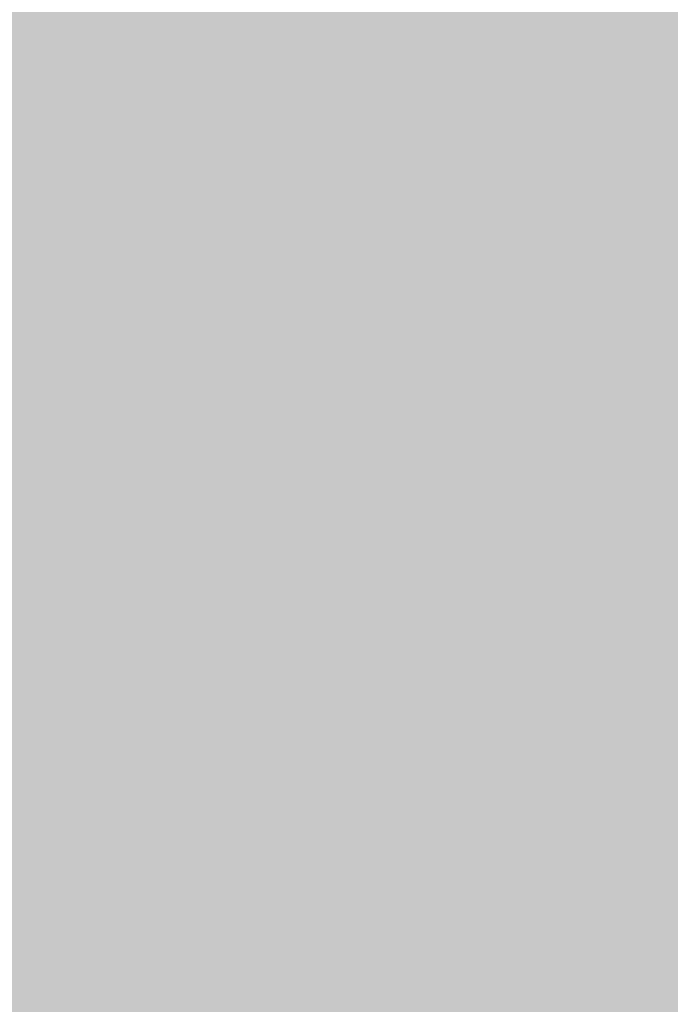
# Model space of a CAD drawing. Units: millimetres. Extents: x 0 to 2267, y 0 to 1823.
# Tile 43 of 256: x 1593.5605 to 1593.7801, y 1226.3857 to 1226.718. Entities that reach past the tile are written whole.
import ezdxf

# ---------------------------------------------------------------- set-up
doc = ezdxf.new("R2010")
doc.units = ezdxf.units.MM
doc.header["$MEASUREMENT"] = 0
doc.layers.add('M-HATC', color=252, linetype='Continuous', lineweight=18)

msp = doc.modelspace()

# ---------------------------------------------------------------- hatches: boundary and pattern name
at = {"layer": 'M-HATC'}
h = msp.add_hatch(color=256, dxfattribs=at)
h.dxf.hatch_style = 1
h.paths.add_polyline_path([(2055.77105, 1603.06204), (1381.08677, 1603.06204), (1381.08677, 1598.06204), (2055.77105, 1598.06204)])
h.paths.add_polyline_path([(2055.77105, 1598.06204), (1381.08677, 1598.06204), (1381.08677, 1593.06204), (2055.77105, 1593.06204)])
h.paths.add_polyline_path([(2051.30737, 1536.76088), (1385.55044, 1536.76088), (1385.55044, 1526.76088), (1387.55044, 1526.76088), (1388.53662, 1525.05276), (1385.33187, 1521.23348), (1385.33187, 1521.22256), (2050.25417, 1522.74913), (2048.32119, 1525.05276), (2049.30737, 1526.76088), (2051.30737, 1526.76088)])
edge = h.paths.add_edge_path()
edge.add_arc((1847.53451, 1379.14917), 135, 222.6030607, 222.8908505, ccw=False)
edge.add_line((1748.16629, 1287.76561), (1683.09212, 1287.76561))
edge.add_arc((1583.7239, 1379.14917), 135, 317.1091495, 317.3969393, ccw=False)
edge.add_arc((1678.9686, 1290.67067), 5, 222.89085, 317.10915, ccw=False)
edge.add_arc((1774.21331, 1379.14917), 135, 222.6030607, 222.8908505, ccw=False)
edge.add_line((1674.84509, 1287.76561), (1609.77092, 1287.76561))
edge.add_arc((1510.4027, 1379.14917), 135, 317.1091495, 317.3969393, ccw=False)
edge.add_arc((1605.6474, 1290.67067), 5, 222.89085, 317.10915, ccw=False)
edge.add_arc((1700.89211, 1379.14917), 135, 222.6030607, 222.8908505, ccw=False)
edge.add_line((1601.52388, 1287.76561), (1536.44972, 1287.76561))
edge.add_arc((1437.08149, 1379.14917), 135, 317.1091495, 317.3969393, ccw=False)
edge.add_arc((1532.3262, 1290.67067), 5, 222.89085, 317.10915, ccw=False)
edge.add_arc((1627.57091, 1379.14917), 135, 222.6030607, 222.8908505, ccw=False)
edge.add_line((1528.20268, 1287.76561), (1505.92891, 1287.76561))
edge.add_spline(control_points=[(1505.92891, 1287.76561), (1504.26224, 1287.76561), (1504.26224, 1282.76561), (1505.92891, 1282.76561)], knot_values=[0, 0, 0, 0, 5, 5, 5, 5], degree=3, periodic=0)
edge.add_line((1505.92891, 1282.76561), (1930.92891, 1282.76561))
edge.add_spline(control_points=[(1930.92891, 1282.76561), (1932.59557, 1282.76561), (1932.59557, 1287.76561), (1930.92891, 1287.76561)], knot_values=[0, 0, 0, 0, 5, 5, 5, 5], degree=3, periodic=0)
edge.add_line((1930.92891, 1287.76561), (1903.05573, 1287.76561))
edge.add_arc((1803.6875, 1379.14917), 135, 317.1091495, 317.3969393, ccw=False)
edge.add_arc((1898.93221, 1290.67067), 5, 222.89085, 317.10915, ccw=False)
edge.add_arc((1994.17691, 1379.14917), 135, 222.6030607, 222.8908505, ccw=False)
edge.add_line((1894.80869, 1287.76561), (1829.73452, 1287.76561))
edge.add_arc((1730.3663, 1379.14917), 135, 317.1091495, 317.3969393, ccw=False)
edge.add_arc((1825.61101, 1290.67067), 5, 222.89085, 317.10915, ccw=False)
edge.add_arc((1920.85571, 1379.14917), 135, 222.6030607, 222.8908505, ccw=False)
edge.add_line((1821.48749, 1287.76561), (1756.41332, 1287.76561))
edge.add_arc((1657.0451, 1379.14917), 135, 317.1091495, 317.3969393, ccw=False)
edge.add_arc((1752.28981, 1290.67067), 5, 222.89085, 317.10915, ccw=False)
edge = h.paths.add_edge_path()
edge.add_spline(control_points=[(1843.42891, 1227.24746), (1845.09557, 1227.24746), (1845.09557, 1232.24746), (1843.42891, 1232.24746)], knot_values=[0, 0, 0, 0, 5, 5, 5, 5], degree=3, periodic=0)
edge.add_line((1843.42891, 1232.24746), (1593.42891, 1232.24746))
edge.add_spline(control_points=[(1593.42891, 1232.24746), (1591.76224, 1232.24746), (1591.76224, 1227.24746), (1593.42891, 1227.24746)], knot_values=[0, 0, 0, 0, 5, 5, 5, 5], degree=3, periodic=0)
edge.add_line((1593.42891, 1227.24746), (1843.42891, 1227.24746))
h.paths.add_polyline_path([(1905.92891, 1127.41706), (1530.92891, 1127.41706, 0.414214), (1520.92891, 1117.41706), (1530.92891, 1117.41706), (1915.92891, 1117.41706, 0.414214)])
edge = h.paths.add_edge_path()
edge.add_arc((1397.08577, 1498.40775), 12.72993, 90.782146, 190.878706, ccw=False)
edge.add_line((1396.912, 1511.13649), (1428.00968, 1511.34875))
edge.add_line((1428.00968, 1511.34875), (1433.00968, 1511.34875))
edge.add_line((1433.00968, 1511.34875), (1434.439, 1511.34875))
edge.add_arc((1419.474, 1498.08041), 20, 41.560995, 74.082109)
edge.add_line((1424.95919, 1517.31353), (1399.93509, 1517.25608))
edge.add_spline(control_points=[(1399.93074, 1517.25607), (1399.88398, 1517.21312), (1399.8328, 1517.16893), (1399.77741, 1517.1236)], knot_values=[11.567499, 11.567499, 11.567499, 11.567499, 11.814249, 11.814249, 11.814249, 11.814249], degree=3, periodic=0)
edge.add_spline(control_points=[(1399.63279, 1517.00986), (1399.58305, 1516.97214), (1399.53072, 1516.93375), (1399.47591, 1516.89474)], knot_values=[11.167718, 11.167718, 11.167718, 11.167718, 11.365188, 11.365188, 11.365188, 11.365188], degree=3, periodic=0)
edge.add_spline(control_points=[(1399.33981, 1516.80007), (1399.15144, 1516.67185), (1398.93836, 1516.5377), (1398.70404, 1516.39942)], knot_values=[10.376405, 10.376405, 10.376405, 10.376405, 11.00994, 11.00994, 11.00994, 11.00994], degree=3, periodic=0)
edge.add_spline(control_points=[(1398.65716, 1516.37187), (1398.57885, 1516.32602), (1398.49825, 1516.27974), (1398.41549, 1516.23309)], knot_values=[10.125175, 10.125175, 10.125175, 10.125175, 10.334406, 10.334406, 10.334406, 10.334406], degree=3, periodic=0)
edge.add_spline(control_points=[(1398.26422, 1516.14874), (1398.19595, 1516.11107), (1398.12634, 1516.07319), (1398.05546, 1516.03513)], knot_values=[9.832246, 9.832246, 9.832246, 9.832246, 9.999658, 9.999658, 9.999658, 9.999658], degree=3, periodic=0)
edge.add_spline(control_points=[(1397.9987, 1516.00476), (1397.73115, 1515.86211), (1397.44602, 1515.71707), (1397.14664, 1515.57138)], knot_values=[9.161808, 9.161808, 9.161808, 9.161808, 9.787769, 9.787769, 9.787769, 9.787769], degree=3, periodic=0)
edge.add_spline(control_points=[(1397.14664, 1515.57138), (1396.84182, 1515.42305), (1396.52223, 1515.27404), (1396.1914, 1515.12621)], knot_values=[8.524455, 8.524455, 8.524455, 8.524455, 9.161808, 9.161808, 9.161808, 9.161808], degree=3, periodic=0)
edge.add_spline(control_points=[(1396.07771, 1515.07565), (1395.98538, 1515.03478), (1395.89222, 1514.99402), (1395.7983, 1514.9534)], knot_values=[8.275193, 8.275193, 8.275193, 8.275193, 8.451726, 8.451726, 8.451726, 8.451726], degree=3, periodic=0)
edge.add_spline(control_points=[(1395.60184, 1514.86912), (1395.49975, 1514.82568), (1395.39685, 1514.78244), (1395.29322, 1514.73944)], knot_values=[7.962917, 7.962917, 7.962917, 7.962917, 8.152764, 8.152764, 8.152764, 8.152764], degree=3, periodic=0)
edge.add_spline(control_points=[(1395.21158, 1514.70568), (1394.82779, 1514.5475), (1394.43452, 1514.39287), (1394.03645, 1514.24422)], knot_values=[7.21254, 7.21254, 7.21254, 7.21254, 7.913148, 7.913148, 7.913148, 7.913148], degree=3, periodic=0)
edge.add_spline(control_points=[(1394.03645, 1514.24422), (1393.70758, 1514.12142), (1393.37544, 1514.0027), (1393.04267, 1513.88945)], knot_values=[6.633733, 6.633733, 6.633733, 6.633733, 7.21254, 7.21254, 7.21254, 7.21254], degree=3, periodic=0)
edge.add_spline(control_points=[(1392.82142, 1513.81499), (1392.71978, 1513.78118), (1392.61815, 1513.74791), (1392.51658, 1513.71521)], knot_values=[6.328796, 6.328796, 6.328796, 6.328796, 6.505493, 6.505493, 6.505493, 6.505493], degree=3, periodic=0)
edge.add_spline(control_points=[(1392.51658, 1513.71521), (1392.31873, 1513.65151), (1392.12116, 1513.59001), (1391.92441, 1513.53098)], knot_values=[5.984605, 5.984605, 5.984605, 5.984605, 6.328796, 6.328796, 6.328796, 6.328796], degree=3, periodic=0)
edge.add_spline(control_points=[(1391.79155, 1513.49146), (1391.31215, 1513.35011), (1390.83842, 1513.22392), (1390.37844, 1513.11711)], knot_values=[5.066697, 5.066697, 5.066697, 5.066697, 5.907055, 5.907055, 5.907055, 5.907055], degree=3, periodic=0)
edge.add_spline(control_points=[(1390.37844, 1513.11711), (1390.17973, 1513.07097), (1389.98359, 1513.02845), (1389.79067, 1512.98988)], knot_values=[4.70367, 4.70367, 4.70367, 4.70367, 5.066695, 5.066695, 5.066695, 5.066695], degree=3, periodic=0)
edge.add_spline(control_points=[(1389.42203, 1512.92036), (1389.24588, 1512.88922), (1389.0729, 1512.86172), (1388.90364, 1512.83814)], knot_values=[4.130571, 4.130571, 4.130571, 4.130571, 4.469816, 4.469816, 4.469816, 4.469816], degree=3, periodic=0)
edge.add_spline(control_points=[(1388.90364, 1512.83814), (1388.59103, 1512.7946), (1388.29108, 1512.76444), (1388.00714, 1512.74941)], knot_values=[3.504031, 3.504031, 3.504031, 3.504031, 4.130571, 4.130571, 4.130571, 4.130571], degree=3, periodic=0)
edge.add_spline(control_points=[(1387.9356, 1512.74593), (1387.85378, 1512.74231), (1387.77334, 1512.73997), (1387.69435, 1512.73898)], knot_values=[3.268866, 3.268866, 3.268866, 3.268866, 3.451164, 3.451164, 3.451164, 3.451164], degree=3, periodic=0)
edge.add_spline(control_points=[(1387.33512, 1512.74426), (1387.20757, 1512.74991), (1387.08472, 1512.7597), (1386.96699, 1512.77385)], knot_values=[2.670686, 2.670686, 2.670686, 2.670686, 2.984, 2.984, 2.984, 2.984], degree=3, periodic=0)
edge.add_spline(control_points=[(1386.83274, 1512.79225), (1386.82093, 1512.79407), (1386.80917, 1512.79594), (1386.79747, 1512.79787)], knot_values=[2.516981, 2.516981, 2.516981, 2.516981, 2.549528, 2.549528, 2.549528, 2.549528], degree=3, periodic=0)
edge.add_spline(control_points=[(1386.45257, 1512.87348), (1386.42573, 1512.88105), (1386.39931, 1512.88895), (1386.3733, 1512.89719)], knot_values=[2.095869, 2.095869, 2.095869, 2.095869, 2.17941, 2.17941, 2.17941, 2.17941], degree=3, periodic=0)
edge.add_spline(control_points=[(1386.06911, 1513.01889), (1386.06338, 1513.02174), (1386.05768, 1513.02463), (1386.05201, 1513.02753)], knot_values=[1.72453, 1.72453, 1.72453, 1.72453, 1.745933, 1.745933, 1.745933, 1.745933], degree=3, periodic=0)
edge.add_arc((1399.474, 1498.08041), 20, 131.824322, 180)
edge.add_arc((1630.33362, 1505.54843), 250.97076, 181.7051759, 236.427975)
edge.add_arc((1605.33992, 1483.30441), 218.7822, 238.660829, 243.3496099)
edge.add_arc((1647.09105, 1510.35917), 262.89859, 183.1298361, 237.8534422, ccw=False)
h.paths.add_polyline_path([(1406.53685, 1391.96444, 0.149382), (1491.55061, 1296.44177, -0.129517)], flags=17)
edge = h.paths.add_edge_path()
edge.add_arc((2037.38381, 1498.08041), 20, 0, 48.265868)
edge.add_spline(control_points=[(2050.69731, 1513.00525), (2050.65121, 1512.98471), (2050.60338, 1512.96554), (2050.55388, 1512.94771)], knot_values=[1.835652, 1.835652, 1.835652, 1.835652, 2.000781, 2.000781, 2.000781, 2.000781], degree=3, periodic=0)
edge.add_spline(control_points=[(2050.46156, 1512.91661), (2050.479, 1512.9221), (2050.49625, 1512.92774), (2050.51332, 1512.93353)], knot_values=[2.045477, 2.045477, 2.045477, 2.045477, 2.101389, 2.101389, 2.101389, 2.101389], degree=3, periodic=0)
edge.add_spline(control_points=[(2050.12896, 1512.83416), (2050.19843, 1512.84734), (2050.26573, 1512.86233), (2050.33075, 1512.87919)], knot_values=[2.237629, 2.237629, 2.237629, 2.237629, 2.435841, 2.435841, 2.435841, 2.435841], degree=3, periodic=0)
edge.add_spline(control_points=[(2050.09463, 1512.82783), (2050.10613, 1512.82989), (2050.11757, 1512.832), (2050.12896, 1512.83416)], knot_values=[2.435841, 2.435841, 2.435841, 2.435841, 2.468321, 2.468321, 2.468321, 2.468321], degree=3, periodic=0)
edge.add_spline(control_points=[(2049.78433, 1512.78511), (2049.85521, 1512.79219), (2049.92435, 1512.80077), (2049.99166, 1512.81088)], knot_values=[2.563852, 2.563852, 2.563852, 2.563852, 2.748541, 2.748541, 2.748541, 2.748541], degree=3, periodic=0)
edge.add_spline(control_points=[(2049.4052, 1512.76169), (2049.5364, 1512.76526), (2049.66292, 1512.77299), (2049.78433, 1512.78511)], knot_values=[2.748541, 2.748541, 2.748541, 2.748541, 3.064882, 3.064882, 3.064882, 3.064882], degree=3, periodic=0)
edge.add_spline(control_points=[(2049.16976, 1512.75968), (2049.23364, 1512.7591), (2049.29654, 1512.7594), (2049.35844, 1512.7606)], knot_values=[3.102309, 3.102309, 3.102309, 3.102309, 3.2503, 3.2503, 3.2503, 3.2503], degree=3, periodic=0)
edge.add_spline(control_points=[(2048.85727, 1512.76911), (2048.96378, 1512.76378), (2049.068, 1512.76061), (2049.16976, 1512.75968)], knot_values=[3.2503, 3.2503, 3.2503, 3.2503, 3.486069, 3.486069, 3.486069, 3.486069], degree=3, periodic=0)
edge.add_spline(control_points=[(2048.69241, 1512.77892), (2048.3729, 1512.80093), (2048.0345, 1512.84106), (2047.68175, 1512.89697)], knot_values=[3.606429, 3.606429, 3.606429, 3.606429, 4.2989, 4.2989, 4.2989, 4.2989], degree=3, periodic=0)
edge.add_spline(control_points=[(2047.68175, 1512.89697), (2047.5458, 1512.91852), (2047.40772, 1512.94241), (2047.26776, 1512.96851)], knot_values=[4.2989, 4.2989, 4.2989, 4.2989, 4.565769, 4.565769, 4.565769, 4.565769], degree=3, periodic=0)
edge.add_spline(control_points=[(2047.26776, 1512.96851), (2047.14494, 1512.99141), (2047.02067, 1513.01601), (2046.89514, 1513.04223)], knot_values=[4.565769, 4.565769, 4.565769, 4.565769, 4.799971, 4.799971, 4.799971, 4.799971], degree=3, periodic=0)
edge.add_spline(control_points=[(2046.89514, 1513.04223), (2046.52865, 1513.11875), (2046.15135, 1513.20899), (2045.7676, 1513.31068)], knot_values=[4.799971, 4.799971, 4.799971, 4.799971, 5.483718, 5.483718, 5.483718, 5.483718], degree=3, periodic=0)
edge.add_spline(control_points=[(2045.7676, 1513.31068), (2045.3724, 1513.41539), (2044.97036, 1513.53225), (2044.56625, 1513.65876)], knot_values=[5.483718, 5.483718, 5.483718, 5.483718, 6.187866, 6.187866, 6.187866, 6.187866], degree=3, periodic=0)
edge.add_spline(control_points=[(2044.56625, 1513.65876), (2044.41491, 1513.70614), (2044.26329, 1513.75487), (2044.11163, 1513.80482)], knot_values=[6.187866, 6.187866, 6.187866, 6.187866, 6.451551, 6.451551, 6.451551, 6.451551], degree=3, periodic=0)
edge.add_spline(control_points=[(2044.11163, 1513.80482), (2043.99666, 1513.84269), (2043.88167, 1513.88126), (2043.76676, 1513.92048)], knot_values=[6.451551, 6.451551, 6.451551, 6.451551, 6.651434, 6.651434, 6.651434, 6.651434], degree=3, periodic=0)
edge.add_spline(control_points=[(2043.76676, 1513.92048), (2043.37157, 1514.05536), (2042.97738, 1514.19789), (2042.58863, 1514.34575)], knot_values=[6.651434, 6.651434, 6.651434, 6.651434, 7.338879, 7.338879, 7.338879, 7.338879], degree=3, periodic=0)
edge.add_spline(control_points=[(2042.58863, 1514.34575), (2042.16431, 1514.50715), (2041.74647, 1514.67491), (2041.34086, 1514.84603)], knot_values=[7.338879, 7.338879, 7.338879, 7.338879, 8.089209, 8.089209, 8.089209, 8.089209], degree=3, periodic=0)
edge.add_spline(control_points=[(2041.34086, 1514.84603), (2041.1028, 1514.94647), (2040.86896, 1515.04806), (2040.64049, 1515.1502)], knot_values=[8.089209, 8.089209, 8.089209, 8.089209, 8.529587, 8.529587, 8.529587, 8.529587], degree=3, periodic=0)
edge.add_spline(control_points=[(2040.50999, 1515.20887), (2040.08238, 1515.40218), (2039.67475, 1515.59705), (2039.29495, 1515.78939)], knot_values=[8.613818, 8.613818, 8.613818, 8.613818, 9.44571, 9.44571, 9.44571, 9.44571], degree=3, periodic=0)
edge.add_spline(control_points=[(2039.29495, 1515.78939), (2039.0618, 1515.90746), (2038.83914, 1516.02458), (2038.62878, 1516.1398)], knot_values=[9.44571, 9.44571, 9.44571, 9.44571, 9.956404, 9.956404, 9.956404, 9.956404], degree=3, periodic=0)
edge.add_spline(control_points=[(2038.62878, 1516.1398), (2038.51874, 1516.20007), (2038.41207, 1516.25982), (2038.30903, 1516.31891)], knot_values=[9.956404, 9.956404, 9.956404, 9.956404, 10.223542, 10.223542, 10.223542, 10.223542], degree=3, periodic=0)
edge.add_spline(control_points=[(2038.30903, 1516.31891), (2038.21377, 1516.37354), (2038.12161, 1516.42762), (2038.03275, 1516.48102)], knot_values=[10.223542, 10.223542, 10.223542, 10.223542, 10.47051, 10.47051, 10.47051, 10.47051], degree=3, periodic=0)
edge.add_spline(control_points=[(2038.03275, 1516.48102), (2037.78552, 1516.62961), (2037.56388, 1516.77304), (2037.37225, 1516.909)], knot_values=[10.47051, 10.47051, 10.47051, 10.47051, 11.15767, 11.15767, 11.15767, 11.15767], degree=3, periodic=0)
edge.add_spline(control_points=[(2037.37225, 1516.909), (2037.27893, 1516.9752), (2037.19274, 1517.03963), (2037.11417, 1517.10203)], knot_values=[11.15767, 11.15767, 11.15767, 11.15767, 11.49227, 11.49227, 11.49227, 11.49227], degree=3, periodic=0)
edge.add_spline(control_points=[(2036.85638, 1517.32585), (2036.91481, 1517.26923), (2036.98143, 1517.21027), (2037.05573, 1517.14922)], knot_values=[11.577341, 11.577341, 11.577341, 11.577341, 11.91035, 11.91035, 11.91035, 11.91035], degree=3, periodic=0)
edge.add_spline(control_points=[(2036.80739, 1517.37475), (2036.82301, 1517.35865), (2036.83935, 1517.34235), (2036.85638, 1517.32585)], knot_values=[11.91035, 11.91035, 11.91035, 11.91035, 12.007402, 12.007402, 12.007402, 12.007402], degree=3, periodic=0)
edge.add_spline(control_points=[(2036.70167, 1517.494), (2036.71042, 1517.48299), (2036.71958, 1517.47185), (2036.72913, 1517.4606)], knot_values=[12.184155, 12.184155, 12.184155, 12.184155, 12.255409, 12.255409, 12.255409, 12.255409], degree=3, periodic=0)
edge.add_spline(control_points=[(2036.6159, 1517.6205), (2036.61998, 1517.61304), (2036.6243, 1517.6055), (2036.62885, 1517.59789)], knot_values=[12.487913, 12.487913, 12.487913, 12.487913, 12.541035, 12.541035, 12.541035, 12.541035], degree=3, periodic=0)
edge.add_spline(control_points=[(2036.56349, 1517.78599), (2036.56372, 1517.77936), (2036.56423, 1517.77264), (2036.56502, 1517.76582)], knot_values=[12.911761, 12.911761, 12.911761, 12.911761, 12.968286, 12.968286, 12.968286, 12.968286], degree=3, periodic=0)
edge.add_spline(control_points=[(2036.61663, 1517.93042), (2036.61248, 1517.92586), (2036.60857, 1517.92121), (2036.60491, 1517.91648)], knot_values=[13.382527, 13.382527, 13.382527, 13.382527, 13.433791, 13.433791, 13.433791, 13.433791], degree=3, periodic=0)
edge.add_spline(control_points=[(2036.74902, 1518.01695), (2036.73613, 1518.0116), (2036.72393, 1518.00601), (2036.71242, 1518.00018)], knot_values=[13.726299, 13.726299, 13.726299, 13.726299, 13.809928, 13.809928, 13.809928, 13.809928], degree=3, periodic=0)
edge.add_spline(control_points=[(2036.86043, 1518.05285), (2036.83863, 1518.04743), (2036.81809, 1518.04156), (2036.79879, 1518.03526)], knot_values=[13.910887, 13.910887, 13.910887, 13.910887, 14.02153, 14.02153, 14.02153, 14.02153], degree=3, periodic=0)
edge.add_line((2036.96387, 1518.08041), (2032.38381, 1518.08041))
edge.add_line((2032.38381, 1518.08041), (2027.38381, 1518.08041))
edge.add_line((2027.38381, 1518.08041), (2022.38381, 1518.08041))
edge.add_line((2022.38381, 1518.08041), (2017.38381, 1518.08041))
edge.add_arc((2017.38381, 1498.08041), 20, 90, 138.439005)
edge.add_line((2002.41881, 1511.34875), (2003.84813, 1511.34875))
edge.add_line((2003.84813, 1511.34875), (2008.84813, 1511.34875))
edge.add_line((2008.84813, 1511.34875), (2039.77204, 1511.13768))
edge.add_arc((2039.77204, 1498.40775), 12.72993, -10.878706, 90, ccw=False)
edge.add_arc((1789.76676, 1510.35917), 262.89859, 302.1465578, 356.8701639, ccw=False)
edge.add_arc((1831.51789, 1483.30441), 218.7822, 296.6503901, 301.339171)
edge.add_arc((1806.52419, 1505.54843), 250.97076, 303.572025, 358.2948241)
h.paths.add_polyline_path([(2030.32096, 1391.96444, -0.129517), (1945.3072, 1296.44177, 0.149382)], flags=17)
edge = h.paths.add_edge_path()
edge.add_spline(control_points=[(2037.2464, 1518.08209), (2037.28977, 1518.08098), (2037.33555, 1518.08041), (2037.3838, 1518.08041)], knot_values=[0.000012, 0.000012, 0.000012, 0.000012, 0.144754, 0.144754, 0.144754, 0.144754], degree=3, periodic=0)
edge.add_line((2037.33571, 1518.08041), (2037.00963, 1518.08041))
edge.add_spline(control_points=[(2037.00963, 1518.08041), (2036.98217, 1518.07678), (2036.95605, 1518.07266), (2036.93124, 1518.06808)], knot_values=[14.13465, 14.13465, 14.13465, 14.13465, 14.247197, 14.247197, 14.247197, 14.247197], degree=3, periodic=0)
edge.add_spline(control_points=[(2036.93124, 1518.06808), (2036.92764, 1518.06741), (2036.92407, 1518.06674), (2036.92053, 1518.06605)], knot_values=[14.118315, 14.118315, 14.118315, 14.118315, 14.13465, 14.13465, 14.13465, 14.13465], degree=3, periodic=0)
edge.add_spline(control_points=[(2036.92053, 1518.06605), (2036.9118, 1518.06436), (2036.90323, 1518.06262), (2036.89484, 1518.06081)], knot_values=[14.078086, 14.078086, 14.078086, 14.078086, 14.118315, 14.118315, 14.118315, 14.118315], degree=3, periodic=0)
edge.add_spline(control_points=[(2036.89484, 1518.06081), (2036.88304, 1518.05827), (2036.87157, 1518.05562), (2036.86043, 1518.05285)], knot_values=[14.02153, 14.02153, 14.02153, 14.02153, 14.078086, 14.078086, 14.078086, 14.078086], degree=3, periodic=0)
edge.add_spline(control_points=[(2036.86043, 1518.05285), (2036.83863, 1518.04743), (2036.81809, 1518.04156), (2036.79879, 1518.03526)], knot_values=[13.910887, 13.910887, 13.910887, 13.910887, 14.02153, 14.02153, 14.02153, 14.02153], degree=3, periodic=0)
edge.add_spline(control_points=[(2036.79879, 1518.03526), (2036.79809, 1518.03504), (2036.7974, 1518.03481), (2036.79671, 1518.03458)], knot_values=[13.906906, 13.906906, 13.906906, 13.906906, 13.910887, 13.910887, 13.910887, 13.910887], degree=3, periodic=0)
edge.add_spline(control_points=[(2036.79671, 1518.03458), (2036.78819, 1518.03178), (2036.77991, 1518.02888), (2036.77187, 1518.02591)], knot_values=[13.857826, 13.857826, 13.857826, 13.857826, 13.906906, 13.906906, 13.906906, 13.906906], degree=3, periodic=0)
edge.add_spline(control_points=[(2036.77187, 1518.02591), (2036.76402, 1518.023), (2036.75641, 1518.02002), (2036.74902, 1518.01695)], knot_values=[13.809928, 13.809928, 13.809928, 13.809928, 13.857826, 13.857826, 13.857826, 13.857826], degree=3, periodic=0)
edge.add_spline(control_points=[(2036.74902, 1518.01695), (2036.73613, 1518.0116), (2036.72393, 1518.00601), (2036.71242, 1518.00018)], knot_values=[13.726299, 13.726299, 13.726299, 13.726299, 13.809928, 13.809928, 13.809928, 13.809928], degree=3, periodic=0)
edge.add_spline(control_points=[(2036.71242, 1518.00018), (2036.71211, 1518.00002), (2036.71179, 1517.99986), (2036.71147, 1517.99969)], knot_values=[13.723993, 13.723993, 13.723993, 13.723993, 13.726299, 13.726299, 13.726299, 13.726299], degree=3, periodic=0)
edge.add_spline(control_points=[(2036.71147, 1517.99969), (2036.70634, 1517.99708), (2036.70134, 1517.99441), (2036.69648, 1517.9917)], knot_values=[13.686536, 13.686536, 13.686536, 13.686536, 13.723993, 13.723993, 13.723993, 13.723993], degree=3, periodic=0)
edge.add_spline(control_points=[(2036.69648, 1517.9917), (2036.6919, 1517.98914), (2036.68744, 1517.98654), (2036.6831, 1517.9839)], knot_values=[13.651251, 13.651251, 13.651251, 13.651251, 13.686536, 13.686536, 13.686536, 13.686536], degree=3, periodic=0)
edge.add_spline(control_points=[(2036.6831, 1517.9839), (2036.67641, 1517.97983), (2036.67001, 1517.97566), (2036.6639, 1517.97139)], knot_values=[13.596804, 13.596804, 13.596804, 13.596804, 13.651251, 13.651251, 13.651251, 13.651251], degree=3, periodic=0)
edge.add_spline(control_points=[(2036.6639, 1517.97139), (2036.66358, 1517.97117), (2036.66326, 1517.97094), (2036.66294, 1517.97072)], knot_values=[13.593956, 13.593956, 13.593956, 13.593956, 13.596804, 13.596804, 13.596804, 13.596804], degree=3, periodic=0)
edge.add_spline(control_points=[(2036.66294, 1517.97072), (2036.6603, 1517.96886), (2036.65771, 1517.96698), (2036.65518, 1517.96509)], knot_values=[13.570322, 13.570322, 13.570322, 13.570322, 13.593956, 13.593956, 13.593956, 13.593956], degree=3, periodic=0)
edge.add_spline(control_points=[(2036.65518, 1517.96509), (2036.65251, 1517.9631), (2036.64991, 1517.96108), (2036.64737, 1517.95905)], knot_values=[13.545477, 13.545477, 13.545477, 13.545477, 13.570322, 13.570322, 13.570322, 13.570322], degree=3, periodic=0)
edge.add_spline(control_points=[(2036.64737, 1517.95905), (2036.64721, 1517.95892), (2036.64705, 1517.9588), (2036.64689, 1517.95867)], knot_values=[13.543931, 13.543931, 13.543931, 13.543931, 13.545477, 13.545477, 13.545477, 13.545477], degree=3, periodic=0)
edge.add_spline(control_points=[(2036.64689, 1517.95867), (2036.64121, 1517.95411), (2036.63582, 1517.94945), (2036.63073, 1517.94468)], knot_values=[13.488237, 13.488237, 13.488237, 13.488237, 13.543931, 13.543931, 13.543931, 13.543931], degree=3, periodic=0)
edge.add_spline(control_points=[(2036.63073, 1517.94468), (2036.62817, 1517.94229), (2036.62569, 1517.93988), (2036.62329, 1517.93744)], knot_values=[13.460307, 13.460307, 13.460307, 13.460307, 13.488237, 13.488237, 13.488237, 13.488237], degree=3, periodic=0)
edge.add_spline(control_points=[(2036.62329, 1517.93744), (2036.62151, 1517.93564), (2036.61978, 1517.93383), (2036.61809, 1517.932)], knot_values=[13.439712, 13.439712, 13.439712, 13.439712, 13.460307, 13.460307, 13.460307, 13.460307], degree=3, periodic=0)
edge.add_spline(control_points=[(2036.61809, 1517.932), (2036.6176, 1517.93147), (2036.61711, 1517.93095), (2036.61663, 1517.93042)], knot_values=[13.433791, 13.433791, 13.433791, 13.433791, 13.439712, 13.439712, 13.439712, 13.439712], degree=3, periodic=0)
edge.add_spline(control_points=[(2036.61663, 1517.93042), (2036.61248, 1517.92586), (2036.60857, 1517.92121), (2036.60491, 1517.91648)], knot_values=[13.382527, 13.382527, 13.382527, 13.382527, 13.433791, 13.433791, 13.433791, 13.433791], degree=3, periodic=0)
edge.add_spline(control_points=[(2036.60491, 1517.91648), (2036.60258, 1517.91347), (2036.60036, 1517.91044), (2036.59824, 1517.90737)], knot_values=[13.350017, 13.350017, 13.350017, 13.350017, 13.382527, 13.382527, 13.382527, 13.382527], degree=3, periodic=0)
edge.add_spline(control_points=[(2036.59824, 1517.90737), (2036.59718, 1517.90585), (2036.59616, 1517.90433), (2036.59515, 1517.90279)], knot_values=[13.333922, 13.333922, 13.333922, 13.333922, 13.350017, 13.350017, 13.350017, 13.350017], degree=3, periodic=0)
edge.add_spline(control_points=[(2036.59515, 1517.90279), (2036.59452, 1517.90183), (2036.5939, 1517.90086), (2036.59329, 1517.89989)], knot_values=[13.323828, 13.323828, 13.323828, 13.323828, 13.333922, 13.333922, 13.333922, 13.333922], degree=3, periodic=0)
edge.add_spline(control_points=[(2036.59329, 1517.89989), (2036.59049, 1517.89545), (2036.5879, 1517.89094), (2036.5855, 1517.88637)], knot_values=[13.277545, 13.277545, 13.277545, 13.277545, 13.323828, 13.323828, 13.323828, 13.323828], degree=3, periodic=0)
edge.add_spline(control_points=[(2036.5855, 1517.88637), (2036.58355, 1517.88267), (2036.58174, 1517.87892), (2036.58006, 1517.87513)], knot_values=[13.240119, 13.240119, 13.240119, 13.240119, 13.277545, 13.277545, 13.277545, 13.277545], degree=3, periodic=0)
edge.add_spline(control_points=[(2036.58006, 1517.87513), (2036.57952, 1517.87393), (2036.579, 1517.87272), (2036.57849, 1517.87151)], knot_values=[13.228211, 13.228211, 13.228211, 13.228211, 13.240119, 13.240119, 13.240119, 13.240119], degree=3, periodic=0)
edge.add_spline(control_points=[(2036.57849, 1517.87151), (2036.57796, 1517.87023), (2036.57744, 1517.86896), (2036.57693, 1517.86767)], knot_values=[13.215717, 13.215717, 13.215717, 13.215717, 13.228211, 13.228211, 13.228211, 13.228211], degree=3, periodic=0)
edge.add_spline(control_points=[(2036.57693, 1517.86767), (2036.57548, 1517.86399), (2036.57414, 1517.86027), (2036.57293, 1517.85651)], knot_values=[13.179847, 13.179847, 13.179847, 13.179847, 13.215717, 13.215717, 13.215717, 13.215717], degree=3, periodic=0)
edge.add_spline(control_points=[(2036.57293, 1517.85651), (2036.5713, 1517.8515), (2036.56989, 1517.84641), (2036.56868, 1517.84126)], knot_values=[13.132017, 13.132017, 13.132017, 13.132017, 13.179847, 13.179847, 13.179847, 13.179847], degree=3, periodic=0)
edge.add_spline(control_points=[(2036.56868, 1517.84126), (2036.56844, 1517.84023), (2036.56821, 1517.8392), (2036.56798, 1517.83817)], knot_values=[13.122482, 13.122482, 13.122482, 13.122482, 13.132017, 13.132017, 13.132017, 13.132017], degree=3, periodic=0)
edge.add_spline(control_points=[(2036.56798, 1517.83817), (2036.56758, 1517.83634), (2036.56721, 1517.8345), (2036.56687, 1517.83266)], knot_values=[13.105592, 13.105592, 13.105592, 13.105592, 13.122482, 13.122482, 13.122482, 13.122482], degree=3, periodic=0)
edge.add_spline(control_points=[(2036.56687, 1517.83266), (2036.56622, 1517.82921), (2036.56567, 1517.82574), (2036.5652, 1517.82223)], knot_values=[13.074063, 13.074063, 13.074063, 13.074063, 13.105592, 13.105592, 13.105592, 13.105592], degree=3, periodic=0)
edge.add_spline(control_points=[(2036.5652, 1517.82223), (2036.5652, 1517.82223), (2036.5652, 1517.82223), (2036.5652, 1517.82223)], knot_values=[13.074043, 13.074043, 13.074043, 13.074043, 13.074063, 13.074063, 13.074063, 13.074063], degree=3, periodic=0)
edge.add_spline(control_points=[(2036.5652, 1517.82223), (2036.56443, 1517.81643), (2036.5639, 1517.81055), (2036.56361, 1517.8046)], knot_values=[13.021884, 13.021884, 13.021884, 13.021884, 13.074043, 13.074043, 13.074043, 13.074043], degree=3, periodic=0)
edge.add_spline(control_points=[(2036.56361, 1517.8046), (2036.56358, 1517.80401), (2036.56356, 1517.80342), (2036.56353, 1517.80283)], knot_values=[13.01674, 13.01674, 13.01674, 13.01674, 13.021884, 13.021884, 13.021884, 13.021884], degree=3, periodic=0)
edge.add_spline(control_points=[(2036.56353, 1517.80283), (2036.56344, 1517.80051), (2036.56338, 1517.79817), (2036.56336, 1517.79582)], knot_values=[12.996438, 12.996438, 12.996438, 12.996438, 13.01674, 13.01674, 13.01674, 13.01674], degree=3, periodic=0)
edge.add_spline(control_points=[(2036.56336, 1517.79582), (2036.56334, 1517.79257), (2036.56338, 1517.78929), (2036.56349, 1517.78599)], knot_values=[12.968286, 12.968286, 12.968286, 12.968286, 12.996438, 12.996438, 12.996438, 12.996438], degree=3, periodic=0)
edge.add_spline(control_points=[(2036.56349, 1517.78599), (2036.56372, 1517.77936), (2036.56423, 1517.77264), (2036.56502, 1517.76582)], knot_values=[12.911761, 12.911761, 12.911761, 12.911761, 12.968286, 12.968286, 12.968286, 12.968286], degree=3, periodic=0)
edge.add_spline(control_points=[(2036.56502, 1517.76582), (2036.56503, 1517.76573), (2036.56504, 1517.76564), (2036.56505, 1517.76555)], knot_values=[12.911017, 12.911017, 12.911017, 12.911017, 12.911761, 12.911761, 12.911761, 12.911761], degree=3, periodic=0)
edge.add_spline(control_points=[(2036.56505, 1517.76555), (2036.56541, 1517.76245), (2036.56583, 1517.75933), (2036.56631, 1517.75619)], knot_values=[12.88528, 12.88528, 12.88528, 12.88528, 12.911017, 12.911017, 12.911017, 12.911017], degree=3, periodic=0)
edge.add_spline(control_points=[(2036.56631, 1517.75619), (2036.56673, 1517.75341), (2036.5672, 1517.75062), (2036.56771, 1517.74782)], knot_values=[12.862519, 12.862519, 12.862519, 12.862519, 12.88528, 12.88528, 12.88528, 12.88528], degree=3, periodic=0)
edge.add_spline(control_points=[(2036.56771, 1517.74782), (2036.56779, 1517.74737), (2036.56788, 1517.74692), (2036.56796, 1517.74647)], knot_values=[12.858885, 12.858885, 12.858885, 12.858885, 12.862519, 12.862519, 12.862519, 12.862519], degree=3, periodic=0)
edge.add_spline(control_points=[(2036.56796, 1517.74647), (2036.5692, 1517.73986), (2036.57069, 1517.73316), (2036.57243, 1517.72638)], knot_values=[12.8053, 12.8053, 12.8053, 12.8053, 12.858885, 12.858885, 12.858885, 12.858885], degree=3, periodic=0)
edge.add_spline(control_points=[(2036.57243, 1517.72638), (2036.5734, 1517.72257), (2036.57446, 1517.71874), (2036.57559, 1517.71488)], knot_values=[12.775176, 12.775176, 12.775176, 12.775176, 12.8053, 12.8053, 12.8053, 12.8053], degree=3, periodic=0)
edge.add_spline(control_points=[(2036.57559, 1517.71488), (2036.57628, 1517.71252), (2036.577, 1517.71015), (2036.57775, 1517.70778)], knot_values=[12.756759, 12.756759, 12.756759, 12.756759, 12.775176, 12.775176, 12.775176, 12.775176], degree=3, periodic=0)
edge.add_spline(control_points=[(2036.57775, 1517.70778), (2036.57808, 1517.70674), (2036.57841, 1517.7057), (2036.57875, 1517.70466)], knot_values=[12.748742, 12.748742, 12.748742, 12.748742, 12.756759, 12.756759, 12.756759, 12.756759], degree=3, periodic=0)
edge.add_spline(control_points=[(2036.57875, 1517.70466), (2036.58082, 1517.6983), (2036.58309, 1517.69187), (2036.58557, 1517.68537)], knot_values=[12.69959, 12.69959, 12.69959, 12.69959, 12.748742, 12.748742, 12.748742, 12.748742], degree=3, periodic=0)
edge.add_spline(control_points=[(2036.58557, 1517.68537), (2036.58762, 1517.68001), (2036.5898, 1517.6746), (2036.59213, 1517.66916)], knot_values=[12.659038, 12.659038, 12.659038, 12.659038, 12.69959, 12.69959, 12.69959, 12.69959], degree=3, periodic=0)
edge.add_spline(control_points=[(2036.59213, 1517.66916), (2036.59397, 1517.66482), (2036.59591, 1517.66047), (2036.59793, 1517.65608)], knot_values=[12.626806, 12.626806, 12.626806, 12.626806, 12.659038, 12.659038, 12.659038, 12.659038], degree=3, periodic=0)
edge.add_spline(control_points=[(2036.59793, 1517.65608), (2036.59839, 1517.65507), (2036.59886, 1517.65406), (2036.59934, 1517.65305)], knot_values=[12.619394, 12.619394, 12.619394, 12.619394, 12.626806, 12.626806, 12.626806, 12.626806], degree=3, periodic=0)
edge.add_spline(control_points=[(2036.59934, 1517.65305), (2036.60435, 1517.64236), (2036.60987, 1517.63151), (2036.61589, 1517.6205)], knot_values=[12.541039, 12.541039, 12.541039, 12.541039, 12.619394, 12.619394, 12.619394, 12.619394], degree=3, periodic=0)
edge.add_spline(control_points=[(2036.61589, 1517.6205), (2036.61589, 1517.6205), (2036.6159, 1517.6205), (2036.6159, 1517.6205)], knot_values=[12.541035, 12.541035, 12.541035, 12.541035, 12.541039, 12.541039, 12.541039, 12.541039], degree=3, periodic=0)
edge.add_spline(control_points=[(2036.6159, 1517.6205), (2036.61998, 1517.61304), (2036.6243, 1517.6055), (2036.62885, 1517.59789)], knot_values=[12.487913, 12.487913, 12.487913, 12.487913, 12.541035, 12.541035, 12.541035, 12.541035], degree=3, periodic=0)
edge.add_spline(control_points=[(2036.62885, 1517.59789), (2036.63261, 1517.5916), (2036.63653, 1517.58526), (2036.64061, 1517.57888)], knot_values=[12.443982, 12.443982, 12.443982, 12.443982, 12.487913, 12.487913, 12.487913, 12.487913], degree=3, periodic=0)
edge.add_spline(control_points=[(2036.64061, 1517.57888), (2036.64144, 1517.57757), (2036.64228, 1517.57626), (2036.64313, 1517.57495)], knot_values=[12.434996, 12.434996, 12.434996, 12.434996, 12.443982, 12.443982, 12.443982, 12.443982], degree=3, periodic=0)
edge.add_spline(control_points=[(2036.64313, 1517.57495), (2036.65306, 1517.55958), (2036.66389, 1517.54394), (2036.6756, 1517.52803)], knot_values=[12.329647, 12.329647, 12.329647, 12.329647, 12.434996, 12.434996, 12.434996, 12.434996], degree=3, periodic=0)
edge.add_spline(control_points=[(2036.6756, 1517.52803), (2036.68385, 1517.51682), (2036.69254, 1517.50548), (2036.70167, 1517.494)], knot_values=[12.255409, 12.255409, 12.255409, 12.255409, 12.329647, 12.329647, 12.329647, 12.329647], degree=3, periodic=0)
edge.add_spline(control_points=[(2036.70167, 1517.494), (2036.71042, 1517.48299), (2036.71958, 1517.47185), (2036.72913, 1517.4606)], knot_values=[12.184155, 12.184155, 12.184155, 12.184155, 12.255409, 12.255409, 12.255409, 12.255409], degree=3, periodic=0)
edge.add_spline(control_points=[(2036.72913, 1517.4606), (2036.74363, 1517.44352), (2036.75904, 1517.42617), (2036.77534, 1517.40855)], knot_values=[12.075961, 12.075961, 12.075961, 12.075961, 12.184155, 12.184155, 12.184155, 12.184155], degree=3, periodic=0)
edge.add_spline(control_points=[(2036.77534, 1517.40855), (2036.77631, 1517.4075), (2036.77729, 1517.40645), (2036.77827, 1517.40539)], knot_values=[12.069502, 12.069502, 12.069502, 12.069502, 12.075961, 12.075961, 12.075961, 12.075961], degree=3, periodic=0)
edge.add_spline(control_points=[(2036.77827, 1517.40539), (2036.78768, 1517.39526), (2036.79739, 1517.38505), (2036.80739, 1517.37475)], knot_values=[12.007402, 12.007402, 12.007402, 12.007402, 12.069502, 12.069502, 12.069502, 12.069502], degree=3, periodic=0)
edge.add_spline(control_points=[(2036.80739, 1517.37475), (2036.82301, 1517.35865), (2036.83935, 1517.34235), (2036.85638, 1517.32585)], knot_values=[11.91035, 11.91035, 11.91035, 11.91035, 12.007402, 12.007402, 12.007402, 12.007402], degree=3, periodic=0)
edge.add_spline(control_points=[(2036.85638, 1517.32585), (2036.91481, 1517.26923), (2036.98143, 1517.21027), (2037.05573, 1517.14922)], knot_values=[11.577341, 11.577341, 11.577341, 11.577341, 11.91035, 11.91035, 11.91035, 11.91035], degree=3, periodic=0)
edge.add_spline(control_points=[(2037.05573, 1517.14922), (2037.07471, 1517.13362), (2037.0942, 1517.11789), (2037.11417, 1517.10203)], knot_values=[11.49227, 11.49227, 11.49227, 11.49227, 11.577341, 11.577341, 11.577341, 11.577341], degree=3, periodic=0)
edge.add_spline(control_points=[(2037.11417, 1517.10203), (2037.19274, 1517.03963), (2037.27893, 1516.9752), (2037.37225, 1516.909)], knot_values=[11.15767, 11.15767, 11.15767, 11.15767, 11.49227, 11.49227, 11.49227, 11.49227], degree=3, periodic=0)
edge.add_spline(control_points=[(2037.37225, 1516.909), (2037.56388, 1516.77304), (2037.78552, 1516.62961), (2038.03275, 1516.48102)], knot_values=[10.47051, 10.47051, 10.47051, 10.47051, 11.15767, 11.15767, 11.15767, 11.15767], degree=3, periodic=0)
edge.add_spline(control_points=[(2038.03275, 1516.48102), (2038.12161, 1516.42762), (2038.21377, 1516.37354), (2038.30903, 1516.31891)], knot_values=[10.223542, 10.223542, 10.223542, 10.223542, 10.47051, 10.47051, 10.47051, 10.47051], degree=3, periodic=0)
edge.add_spline(control_points=[(2038.30903, 1516.31891), (2038.41207, 1516.25982), (2038.51874, 1516.20007), (2038.62878, 1516.1398)], knot_values=[9.956404, 9.956404, 9.956404, 9.956404, 10.223542, 10.223542, 10.223542, 10.223542], degree=3, periodic=0)
edge.add_spline(control_points=[(2038.62878, 1516.1398), (2038.83914, 1516.02458), (2039.0618, 1515.90746), (2039.29495, 1515.78939)], knot_values=[9.44571, 9.44571, 9.44571, 9.44571, 9.956404, 9.956404, 9.956404, 9.956404], degree=3, periodic=0)
edge.add_spline(control_points=[(2039.29495, 1515.78939), (2039.67475, 1515.59705), (2040.08238, 1515.40218), (2040.50999, 1515.20887)], knot_values=[8.613818, 8.613818, 8.613818, 8.613818, 9.44571, 9.44571, 9.44571, 9.44571], degree=3, periodic=0)
edge.add_spline(control_points=[(2040.50999, 1515.20887), (2040.55329, 1515.1893), (2040.59679, 1515.16974), (2040.64049, 1515.1502)], knot_values=[8.529587, 8.529587, 8.529587, 8.529587, 8.613818, 8.613818, 8.613818, 8.613818], degree=3, periodic=0)
edge.add_spline(control_points=[(2040.64049, 1515.1502), (2040.86896, 1515.04806), (2041.1028, 1514.94647), (2041.34086, 1514.84603)], knot_values=[8.089209, 8.089209, 8.089209, 8.089209, 8.529587, 8.529587, 8.529587, 8.529587], degree=3, periodic=0)
edge.add_spline(control_points=[(2041.34086, 1514.84603), (2041.74647, 1514.67491), (2042.16431, 1514.50715), (2042.58863, 1514.34575)], knot_values=[7.338879, 7.338879, 7.338879, 7.338879, 8.089209, 8.089209, 8.089209, 8.089209], degree=3, periodic=0)
edge.add_spline(control_points=[(2042.58863, 1514.34575), (2042.97738, 1514.19789), (2043.37157, 1514.05536), (2043.76676, 1513.92048)], knot_values=[6.651434, 6.651434, 6.651434, 6.651434, 7.338879, 7.338879, 7.338879, 7.338879], degree=3, periodic=0)
edge.add_spline(control_points=[(2043.76676, 1513.92048), (2043.88167, 1513.88126), (2043.99666, 1513.84269), (2044.11163, 1513.80482)], knot_values=[6.451551, 6.451551, 6.451551, 6.451551, 6.651434, 6.651434, 6.651434, 6.651434], degree=3, periodic=0)
edge.add_spline(control_points=[(2044.11163, 1513.80482), (2044.26329, 1513.75487), (2044.41491, 1513.70614), (2044.56625, 1513.65876)], knot_values=[6.187866, 6.187866, 6.187866, 6.187866, 6.451551, 6.451551, 6.451551, 6.451551], degree=3, periodic=0)
edge.add_spline(control_points=[(2044.56625, 1513.65876), (2044.97036, 1513.53225), (2045.3724, 1513.41539), (2045.7676, 1513.31068)], knot_values=[5.483718, 5.483718, 5.483718, 5.483718, 6.187866, 6.187866, 6.187866, 6.187866], degree=3, periodic=0)
edge.add_spline(control_points=[(2045.7676, 1513.31068), (2046.15135, 1513.20899), (2046.52865, 1513.11875), (2046.89514, 1513.04223)], knot_values=[4.799971, 4.799971, 4.799971, 4.799971, 5.483718, 5.483718, 5.483718, 5.483718], degree=3, periodic=0)
edge.add_spline(control_points=[(2046.89514, 1513.04223), (2047.02067, 1513.01601), (2047.14494, 1512.99141), (2047.26776, 1512.96851)], knot_values=[4.565769, 4.565769, 4.565769, 4.565769, 4.799971, 4.799971, 4.799971, 4.799971], degree=3, periodic=0)
edge.add_spline(control_points=[(2047.26776, 1512.96851), (2047.40772, 1512.94241), (2047.5458, 1512.91852), (2047.68175, 1512.89697)], knot_values=[4.2989, 4.2989, 4.2989, 4.2989, 4.565769, 4.565769, 4.565769, 4.565769], degree=3, periodic=0)
edge.add_spline(control_points=[(2047.68175, 1512.89697), (2048.0345, 1512.84106), (2048.3729, 1512.80093), (2048.69241, 1512.77892)], knot_values=[3.606429, 3.606429, 3.606429, 3.606429, 4.2989, 4.2989, 4.2989, 4.2989], degree=3, periodic=0)
edge.add_spline(control_points=[(2048.69241, 1512.77892), (2048.74794, 1512.7751), (2048.8029, 1512.77182), (2048.85727, 1512.76911)], knot_values=[3.486069, 3.486069, 3.486069, 3.486069, 3.606429, 3.606429, 3.606429, 3.606429], degree=3, periodic=0)
edge.add_spline(control_points=[(2048.85727, 1512.76911), (2048.96378, 1512.76378), (2049.068, 1512.76061), (2049.16976, 1512.75968)], knot_values=[3.2503, 3.2503, 3.2503, 3.2503, 3.486069, 3.486069, 3.486069, 3.486069], degree=3, periodic=0)
edge.add_spline(control_points=[(2049.16976, 1512.75968), (2049.23364, 1512.7591), (2049.29654, 1512.7594), (2049.35844, 1512.7606)], knot_values=[3.102309, 3.102309, 3.102309, 3.102309, 3.2503, 3.2503, 3.2503, 3.2503], degree=3, periodic=0)
edge.add_spline(control_points=[(2049.35844, 1512.7606), (2049.37409, 1512.76091), (2049.38968, 1512.76127), (2049.4052, 1512.76169)], knot_values=[3.064882, 3.064882, 3.064882, 3.064882, 3.102309, 3.102309, 3.102309, 3.102309], degree=3, periodic=0)
edge.add_spline(control_points=[(2049.4052, 1512.76169), (2049.5364, 1512.76526), (2049.66292, 1512.77299), (2049.78433, 1512.78511)], knot_values=[2.748541, 2.748541, 2.748541, 2.748541, 3.064882, 3.064882, 3.064882, 3.064882], degree=3, periodic=0)
edge.add_spline(control_points=[(2049.78433, 1512.78511), (2049.85521, 1512.79219), (2049.92435, 1512.80077), (2049.99166, 1512.81088)], knot_values=[2.563852, 2.563852, 2.563852, 2.563852, 2.748541, 2.748541, 2.748541, 2.748541], degree=3, periodic=0)
edge.add_spline(control_points=[(2049.99166, 1512.81088), (2050.02648, 1512.81612), (2050.0608, 1512.82177), (2050.09463, 1512.82783)], knot_values=[2.468321, 2.468321, 2.468321, 2.468321, 2.563852, 2.563852, 2.563852, 2.563852], degree=3, periodic=0)
edge.add_spline(control_points=[(2050.09463, 1512.82783), (2050.10613, 1512.82989), (2050.11757, 1512.832), (2050.12896, 1512.83416)], knot_values=[2.435841, 2.435841, 2.435841, 2.435841, 2.468321, 2.468321, 2.468321, 2.468321], degree=3, periodic=0)
edge.add_spline(control_points=[(2050.12896, 1512.83416), (2050.19843, 1512.84734), (2050.26573, 1512.86233), (2050.33075, 1512.87919)], knot_values=[2.237629, 2.237629, 2.237629, 2.237629, 2.435841, 2.435841, 2.435841, 2.435841], degree=3, periodic=0)
edge.add_spline(control_points=[(2050.33075, 1512.87919), (2050.37544, 1512.89077), (2050.41906, 1512.90324), (2050.46156, 1512.91661)], knot_values=[2.101389, 2.101389, 2.101389, 2.101389, 2.237629, 2.237629, 2.237629, 2.237629], degree=3, periodic=0)
edge.add_spline(control_points=[(2050.46156, 1512.91661), (2050.479, 1512.9221), (2050.49625, 1512.92774), (2050.51332, 1512.93353)], knot_values=[2.045477, 2.045477, 2.045477, 2.045477, 2.101389, 2.101389, 2.101389, 2.101389], degree=3, periodic=0)
edge.add_spline(control_points=[(2050.51332, 1512.93353), (2050.52696, 1512.93816), (2050.54048, 1512.94288), (2050.55388, 1512.94771)], knot_values=[2.000781, 2.000781, 2.000781, 2.000781, 2.045477, 2.045477, 2.045477, 2.045477], degree=3, periodic=0)
edge.add_spline(control_points=[(2050.55388, 1512.94771), (2050.60338, 1512.96554), (2050.65121, 1512.98471), (2050.69731, 1513.00525)], knot_values=[1.835652, 1.835652, 1.835652, 1.835652, 2.000781, 2.000781, 2.000781, 2.000781], degree=3, periodic=0)
edge.add_arc((2037.38381, 1498.08041), 20, 48.265868, 90.129934)
edge = h.paths.add_edge_path(flags=16)
edge.add_spline(control_points=[(1386.13885, 1512.98591), (1388.91997, 1511.73946), (1398.03873, 1515.51866), (1399.93074, 1517.25607)], knot_values=[1.831046, 1.831046, 1.831046, 1.831046, 11.814249, 11.814249, 11.814249, 11.814249], degree=3, periodic=0)
edge.add_line((1399.93074, 1517.25607), (1393.74348, 1517.24186))
edge.add_arc((1399.474, 1498.08041), 20, 106.650105, 131.817301)
h = msp.add_hatch(color=256, dxfattribs=at)
h.dxf.hatch_style = 1
h.paths.add_polyline_path([(2042.88863, 1580.17963), (2055.77105, 1593.06204), (1381.08677, 1593.06204), (1393.96918, 1580.17963), (1374.08597, 1560.29642), (2062.77184, 1560.29642)])
h.paths.add_polyline_path([(1843.42891, 1201.32971), (1843.42891, 1227.24746), (1593.42891, 1227.24746), (1593.42891, 1201.32971, -0.228274), (1574.59893, 1162.23457), (1530.92891, 1127.41706), (1905.92891, 1127.41706), (1862.25888, 1162.23457, -0.228274)])

doc.saveas('drawing.dxf')
